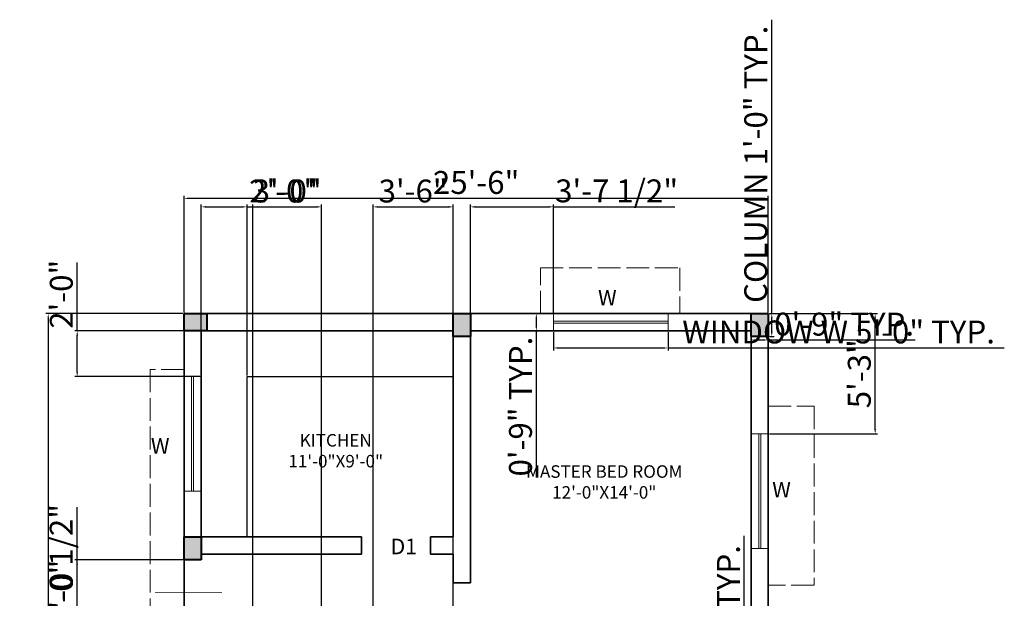
# Model space of a CAD drawing. Units: inches. Extents: x 27449 to 27965, y 46348 to 47103.
# Tile 2 of 2: x 27449 to 27965, y 46800 to 47103. Entities that reach past the tile are written whole.
import ezdxf

# ---------------------------------------------------------------- set-up
doc = ezdxf.new("R2010")
doc.units = ezdxf.units.IN
doc.linetypes.add('ACAD_ISO02W100', pattern=[15, 12, -3])
for name, color, linetype, lineweight in [('A-ANNO-DIMS', 2, 'Continuous', 18), ('A-ANNO-SYMB', 7, 'Continuous', 18), ('A-ANNO-TEXT', 7, 'Continuous', 18), ('A-AREA-IDEN', 7, 'Continuous', 20), ('A-COLS', 7, 'Continuous', 40), ('A-FLOR-FIXT', 9, 'Continuous', 25), ('A-GLAZ', 4, 'Continuous', 20), ('A-GLAZ-OVHD', 8, 'ACAD_ISO02W100', 13), ('A-WALL', 7, 'Continuous', 35)]:
    doc.layers.add(name, color=color, linetype=linetype, lineweight=lineweight)
doc.styles.get("Standard").update_dxf_attribs({"font": 'arial.ttf'})
doc.dimstyles.new('ISO-25', dxfattribs={"dimtxt": 12, "dimasz": 2.5, "dimexe": 1.25, "dimexo": 0.625, "dimtad": 1, "dimlunit": 3, "dimtxsty": 'Standard', "dimcen": 2.5, "dimadec": 0, "dimazin": 0, "dimtfac": 1, "dimtmove": 0, "dimatfit": 3, "dimfxl": 1, "dimarcsym": 0})

# ---------------------------------------------------------------- blocks, each defined once
blk = doc.blocks.new('*D1')
at = {"layer": 'A-ANNO-DIMS', "color": 0, "lineweight": -2, "transparency": 16777216}
for p, q in [((27534.79, 46948.86), (27463.05, 46948.86)), ((27464.3, 46946.36), (27464.3, 46393.36)), ((27534.79, 46390.86), (27463.05, 46390.86))]:
    blk.add_line(p, q, dxfattribs=at)
at = {"layer": 'A-ANNO-DIMS', "color": 0, "transparency": 16777216}
for points in [[(27463.88, 46946.36), (27464.71, 46946.36), (27464.3, 46948.86)], [(27463.88, 46393.36), (27464.71, 46393.36), (27464.3, 46390.86)]]:
    blk.add_solid(points, dxfattribs=at)
at = {"layer": 'Defpoints', "color": 0, "transparency": 16777216}
for p in [(27535.42, 46948.86), (27464.3, 46390.86), (27535.42, 46390.86)]:
    blk.add_point(p, dxfattribs=at)
at = {"layer": 'A-ANNO-DIMS', "color": 0, "transparency": 16777216, "insert": (27457.54, 46669.86), "char_height": 12, "attachment_point": 5, "rotation": 90}
blk.add_mtext('46\'-6"', dxfattribs=at)
blk = doc.blocks.new('*D2')
at = {"layer": 'A-ANNO-DIMS', "color": 0, "lineweight": -2, "transparency": 16777216}
for p, q in [((27535.42, 46949.49), (27535.42, 47010.55)), ((27841.42, 46949.49), (27841.42, 47010.55)), ((27537.92, 47009.3), (27838.92, 47009.3))]:
    blk.add_line(p, q, dxfattribs=at)
at = {"layer": 'A-ANNO-DIMS', "color": 0, "transparency": 16777216}
for points in [[(27537.92, 47009.72), (27537.92, 47008.88), (27535.42, 47009.3)], [(27838.92, 47009.72), (27838.92, 47008.88), (27841.42, 47009.3)]]:
    blk.add_solid(points, dxfattribs=at)
at = {"layer": 'Defpoints', "color": 0, "transparency": 16777216}
for p in [(27841.42, 47009.3), (27535.42, 46948.86), (27841.42, 46948.86)]:
    blk.add_point(p, dxfattribs=at)
at = {"layer": 'A-ANNO-DIMS', "color": 0, "transparency": 16777216, "insert": (27688.42, 47016.05), "char_height": 12, "attachment_point": 5}
blk.add_mtext('25\'-6"', dxfattribs=at)
blk = doc.blocks.new('WIN-W-60IN')
for p, q in [((0, 60), (9, 60)), ((0, 0), (0, 60)), ((4, 0), (4, 60)), ((5, 0), (5, 60)), ((9, 60), (9, 0)), ((9, 0), (0, 0))]:
    blk.add_line(p, q)
blk = doc.blocks.new('COL-9X12IN')
h = blk.add_hatch(color=256)
h.dxf.hatch_style = 1
h.paths.add_polyline_path([(9, 12), (0, 12), (0, 0), (9, 0)])
for p, q in [((0, 12), (9, 12)), ((0, 0), (0, 12)), ((9, 12), (9, 0)), ((9, 0), (0, 0))]:
    blk.add_line(p, q)
blk = doc.blocks.new('ENTRY-ARROW')
blk.add_lwpolyline([(0, 0, 0.5, 0.5, 0), (0, 22.23, 5, 0, 0), (0, 35.55, 0, 0, 0)], format="xyseb")
blk = doc.blocks.new('*D7')
at = {"layer": 'A-ANNO-DIMS', "color": 0, "lineweight": -2, "transparency": 16777216}
for p, q in [((27843.22, 46948.86), (27843.22, 47102.92)), ((27842.04, 46948.86), (27844.47, 46948.86)), ((27843.22, 46939.36), (27843.22, 46946.36)), ((27842.04, 46936.86), (27844.47, 46936.86))]:
    blk.add_line(p, q, dxfattribs=at)
at = {"layer": 'A-ANNO-DIMS', "color": 0, "transparency": 16777216}
for points in [[(27842.8, 46946.36), (27843.64, 46946.36), (27843.22, 46948.86)], [(27842.8, 46939.36), (27843.64, 46939.36), (27843.22, 46936.86)]]:
    blk.add_solid(points, dxfattribs=at)
at = {"layer": 'Defpoints', "color": 0, "transparency": 16777216}
for p in [(27841.42, 46948.86), (27843.22, 46948.86), (27841.42, 46936.86)]:
    blk.add_point(p, dxfattribs=at)
at = {"layer": 'A-ANNO-DIMS', "color": 0, "transparency": 16777216, "insert": (27836.39, 47027.14), "char_height": 12, "attachment_point": 5, "rotation": 90}
blk.add_mtext('COLUMN 1\'-0" TYP.', dxfattribs=at)
blk = doc.blocks.new('*D8')
at = {"layer": 'A-ANNO-DIMS', "color": 0, "lineweight": -2, "transparency": 16777216}
for p, q in [((27832.42, 46936.24), (27832.42, 46933.81)), ((27834.92, 46935.06), (27838.92, 46935.06)), ((27841.42, 46936.24), (27841.42, 46933.81)), ((27841.42, 46935.06), (27918.32, 46935.06))]:
    blk.add_line(p, q, dxfattribs=at)
at = {"layer": 'A-ANNO-DIMS', "color": 0, "transparency": 16777216}
for points in [[(27834.92, 46935.48), (27834.92, 46934.65), (27832.42, 46935.06)], [(27838.92, 46935.48), (27838.92, 46934.65), (27841.42, 46935.06)]]:
    blk.add_solid(points, dxfattribs=at)
at = {"layer": 'Defpoints', "color": 0, "transparency": 16777216}
for p in [(27832.42, 46936.86), (27841.42, 46936.86), (27841.42, 46935.06)]:
    blk.add_point(p, dxfattribs=at)
at = {"layer": 'A-ANNO-DIMS', "color": 0, "transparency": 16777216, "insert": (27881.12, 46941.81), "char_height": 12, "attachment_point": 5}
blk.add_mtext('0\'-9" TYP.', dxfattribs=at)
blk = doc.blocks.new('*D9')
at = {"layer": 'A-ANNO-DIMS', "color": 0, "lineweight": -2, "transparency": 16777216}
for p, q in [((27728.92, 46939.24), (27728.92, 46929.61)), ((27788.92, 46939.24), (27788.92, 46929.61)), ((27731.42, 46930.86), (27786.42, 46930.86)), ((27788.92, 46930.86), (27965, 46930.86))]:
    blk.add_line(p, q, dxfattribs=at)
at = {"layer": 'A-ANNO-DIMS', "color": 0, "transparency": 16777216}
for points in [[(27731.42, 46931.28), (27731.42, 46930.45), (27728.92, 46930.86)], [(27786.42, 46931.28), (27786.42, 46930.45), (27788.92, 46930.86)]]:
    blk.add_solid(points, dxfattribs=at)
at = {"layer": 'Defpoints', "color": 0, "transparency": 16777216}
for p in [(27728.92, 46939.86), (27788.92, 46939.86), (27788.92, 46930.86)]:
    blk.add_point(p, dxfattribs=at)
at = {"layer": 'A-ANNO-DIMS', "color": 0, "transparency": 16777216, "insert": (27878.21, 46937.7), "char_height": 12, "attachment_point": 5}
blk.add_mtext('WINDOW W 5\'-0" TYP.', dxfattribs=at)
blk = doc.blocks.new('*D10')
at = {"layer": 'A-ANNO-DIMS', "color": 0, "lineweight": -2, "transparency": 16777216}
for p, q in [((27728.29, 46948.86), (27718.67, 46948.86)), ((27719.92, 46946.36), (27719.92, 46942.36)), ((27728.29, 46939.86), (27718.67, 46939.86)), ((27719.92, 46939.86), (27719.92, 46862.97))]:
    blk.add_line(p, q, dxfattribs=at)
at = {"layer": 'A-ANNO-DIMS', "color": 0, "transparency": 16777216}
for points in [[(27719.5, 46946.36), (27720.34, 46946.36), (27719.92, 46948.86)], [(27719.5, 46942.36), (27720.34, 46942.36), (27719.92, 46939.86)]]:
    blk.add_solid(points, dxfattribs=at)
at = {"layer": 'Defpoints', "color": 0, "transparency": 16777216}
for p in [(27728.92, 46948.86), (27719.92, 46939.86), (27728.92, 46939.86)]:
    blk.add_point(p, dxfattribs=at)
at = {"layer": 'A-ANNO-DIMS', "color": 0, "transparency": 16777216, "insert": (27713.17, 46900.16), "char_height": 12, "attachment_point": 5, "rotation": 90}
blk.add_mtext('0\'-9" TYP.', dxfattribs=at)
blk = doc.blocks.new('*D11')
at = {"layer": 'A-ANNO-DIMS', "color": 0, "lineweight": -2, "transparency": 16777216}
for p, q in [((27828.82, 46689.61), (27828.82, 46832.34)), ((27831.79, 46689.61), (27827.57, 46689.61)), ((27828.82, 46668.11), (27828.82, 46687.11)), ((27831.79, 46665.61), (27827.57, 46665.61))]:
    blk.add_line(p, q, dxfattribs=at)
at = {"layer": 'A-ANNO-DIMS', "color": 0, "transparency": 16777216}
for points in [[(27828.4, 46687.11), (27829.24, 46687.11), (27828.82, 46689.61)], [(27828.4, 46668.11), (27829.24, 46668.11), (27828.82, 46665.61)]]:
    blk.add_solid(points, dxfattribs=at)
at = {"layer": 'Defpoints', "color": 0, "transparency": 16777216}
for p in [(27828.82, 46689.61), (27832.42, 46689.61), (27832.42, 46665.61)]:
    blk.add_point(p, dxfattribs=at)
at = {"layer": 'A-ANNO-DIMS', "color": 0, "transparency": 16777216, "insert": (27822.07, 46762.22), "char_height": 12, "attachment_point": 5, "rotation": 90}
blk.add_mtext('VENT V 2\'-0" TYP.', dxfattribs=at)
blk = doc.blocks.new('*D16')
at = {"layer": 'A-ANNO-DIMS', "color": 0, "lineweight": -2, "transparency": 16777216}
for p, q in [((27479.47, 46783.86), (27479.47, 46847.47)), ((27534.79, 46783.86), (27478.22, 46783.86)), ((27479.47, 46749.86), (27479.47, 46781.36)), ((27534.79, 46747.36), (27478.22, 46747.36))]:
    blk.add_line(p, q, dxfattribs=at)
at = {"layer": 'A-ANNO-DIMS', "color": 0, "transparency": 16777216}
for points in [[(27479.05, 46781.36), (27479.89, 46781.36), (27479.47, 46783.86)], [(27479.05, 46749.86), (27479.89, 46749.86), (27479.47, 46747.36)]]:
    blk.add_solid(points, dxfattribs=at)
at = {"layer": 'Defpoints', "color": 0, "transparency": 16777216}
for p in [(27479.47, 46783.86), (27535.42, 46783.86), (27535.42, 46747.36)]:
    blk.add_point(p, dxfattribs=at)
at = {"layer": 'A-ANNO-DIMS', "color": 0, "transparency": 16777216, "insert": (27472.64, 46816.91), "char_height": 12, "attachment_point": 5, "rotation": 90}
blk.add_mtext('3\'-0 1/2"', dxfattribs=at)
blk = doc.blocks.new('*D17')
at = {"layer": 'A-ANNO-DIMS', "color": 0, "lineweight": -2, "transparency": 16777216}
for p, q in [((27534.79, 46819.86), (27478.22, 46819.86)), ((27479.47, 46786.36), (27479.47, 46817.36)), ((27534.79, 46783.86), (27478.22, 46783.86))]:
    blk.add_line(p, q, dxfattribs=at)
at = {"layer": 'A-ANNO-DIMS', "color": 0, "transparency": 16777216}
for points in [[(27479.05, 46817.36), (27479.89, 46817.36), (27479.47, 46819.86)], [(27479.05, 46786.36), (27479.89, 46786.36), (27479.47, 46783.86)]]:
    blk.add_solid(points, dxfattribs=at)
at = {"layer": 'Defpoints', "color": 0, "transparency": 16777216}
for p in [(27479.47, 46819.86), (27535.42, 46819.86), (27535.42, 46783.86)]:
    blk.add_point(p, dxfattribs=at)
at = {"layer": 'A-ANNO-DIMS', "color": 0, "transparency": 16777216, "insert": (27472.71, 46801.86), "char_height": 12, "attachment_point": 5, "rotation": 90}
blk.add_mtext('3\'-0"', dxfattribs=at)
blk = doc.blocks.new('*D18')
at = {"layer": 'A-ANNO-DIMS', "color": 0, "lineweight": -2, "transparency": 16777216}
for p, q in [((27479.47, 46939.86), (27479.47, 46975.72)), ((27543.79, 46939.86), (27478.22, 46939.86)), ((27479.47, 46918.36), (27479.47, 46937.36)), ((27543.79, 46915.86), (27478.22, 46915.86))]:
    blk.add_line(p, q, dxfattribs=at)
at = {"layer": 'A-ANNO-DIMS', "color": 0, "transparency": 16777216}
for points in [[(27479.05, 46937.36), (27479.89, 46937.36), (27479.47, 46939.86)], [(27479.05, 46918.36), (27479.89, 46918.36), (27479.47, 46915.86)]]:
    blk.add_solid(points, dxfattribs=at)
at = {"layer": 'Defpoints', "color": 0, "transparency": 16777216}
for p in [(27479.47, 46939.86), (27544.42, 46939.86), (27544.42, 46915.86)]:
    blk.add_point(p, dxfattribs=at)
at = {"layer": 'A-ANNO-DIMS', "color": 0, "transparency": 16777216, "insert": (27472.72, 46959.04), "char_height": 12, "attachment_point": 5, "rotation": 90}
blk.add_mtext('2\'-0"', dxfattribs=at)
blk = doc.blocks.new('*D19')
at = {"layer": 'A-ANNO-DIMS', "color": 0, "lineweight": -2, "transparency": 16777216}
for p, q in [((27544.42, 46916.49), (27544.42, 47006.06)), ((27568.42, 46916.49), (27568.42, 47006.06)), ((27546.92, 47004.81), (27565.92, 47004.81)), ((27568.42, 47004.81), (27604.27, 47004.81))]:
    blk.add_line(p, q, dxfattribs=at)
at = {"layer": 'A-ANNO-DIMS', "color": 0, "transparency": 16777216}
for points in [[(27546.92, 47005.23), (27546.92, 47004.4), (27544.42, 47004.81)], [(27565.92, 47005.23), (27565.92, 47004.4), (27568.42, 47004.81)]]:
    blk.add_solid(points, dxfattribs=at)
at = {"layer": 'Defpoints', "color": 0, "transparency": 16777216}
for p in [(27568.42, 47004.81), (27544.42, 46915.86), (27568.42, 46915.86)]:
    blk.add_point(p, dxfattribs=at)
at = {"layer": 'A-ANNO-DIMS', "color": 0, "transparency": 16777216, "insert": (27587.6, 47011.56), "char_height": 12, "attachment_point": 5}
blk.add_mtext('2\'-0"', dxfattribs=at)
blk = doc.blocks.new('*D20')
at = {"layer": 'A-ANNO-DIMS', "color": 0, "lineweight": -2, "transparency": 16777216}
for p, q in [((27571.42, 46498.49), (27571.42, 47006.06)), ((27607.42, 46498.49), (27607.42, 47006.06)), ((27573.92, 47004.81), (27604.92, 47004.81))]:
    blk.add_line(p, q, dxfattribs=at)
at = {"layer": 'A-ANNO-DIMS', "color": 0, "transparency": 16777216}
for points in [[(27573.92, 47005.23), (27573.92, 47004.4), (27571.42, 47004.81)], [(27604.92, 47005.23), (27604.92, 47004.4), (27607.42, 47004.81)]]:
    blk.add_solid(points, dxfattribs=at)
at = {"layer": 'Defpoints', "color": 0, "transparency": 16777216}
for p in [(27607.42, 47004.81), (27571.42, 46497.86), (27607.42, 46497.86)]:
    blk.add_point(p, dxfattribs=at)
at = {"layer": 'A-ANNO-DIMS', "color": 0, "transparency": 16777216, "insert": (27589.42, 47011.57), "char_height": 12, "attachment_point": 5}
blk.add_mtext('3\'-0"', dxfattribs=at)
blk = doc.blocks.new('*D22')
at = {"layer": 'A-ANNO-DIMS', "color": 0, "lineweight": -2, "transparency": 16777216}
for p, q in [((27634.42, 46498.49), (27634.42, 47006.06)), ((27676.42, 46498.49), (27676.42, 47006.06)), ((27636.92, 47004.81), (27673.92, 47004.81))]:
    blk.add_line(p, q, dxfattribs=at)
at = {"layer": 'A-ANNO-DIMS', "color": 0, "transparency": 16777216}
for points in [[(27636.92, 47005.23), (27636.92, 47004.4), (27634.42, 47004.81)], [(27673.92, 47005.23), (27673.92, 47004.4), (27676.42, 47004.81)]]:
    blk.add_solid(points, dxfattribs=at)
at = {"layer": 'Defpoints', "color": 0, "transparency": 16777216}
for p in [(27676.42, 47004.81), (27634.42, 46497.86), (27676.42, 46497.86)]:
    blk.add_point(p, dxfattribs=at)
at = {"layer": 'A-ANNO-DIMS', "color": 0, "transparency": 16777216, "insert": (27655.42, 47011.57), "char_height": 12, "attachment_point": 5}
blk.add_mtext('3\'-6"', dxfattribs=at)
blk = doc.blocks.new('*D27')
at = {"layer": 'A-ANNO-DIMS', "color": 0, "lineweight": -2, "transparency": 16777216}
for p, q in [((27685.42, 46949.49), (27685.42, 47006.06)), ((27728.92, 46949.49), (27728.92, 47006.06)), ((27687.92, 47004.81), (27726.42, 47004.81)), ((27728.92, 47004.81), (27792.52, 47004.81))]:
    blk.add_line(p, q, dxfattribs=at)
at = {"layer": 'A-ANNO-DIMS', "color": 0, "transparency": 16777216}
for points in [[(27687.92, 47005.23), (27687.92, 47004.4), (27685.42, 47004.81)], [(27726.42, 47005.23), (27726.42, 47004.4), (27728.92, 47004.81)]]:
    blk.add_solid(points, dxfattribs=at)
at = {"layer": 'Defpoints', "color": 0, "transparency": 16777216}
for p in [(27728.92, 47004.81), (27685.42, 46948.86), (27728.92, 46948.86)]:
    blk.add_point(p, dxfattribs=at)
at = {"layer": 'A-ANNO-DIMS', "color": 0, "transparency": 16777216, "insert": (27761.97, 47011.65), "char_height": 12, "attachment_point": 5}
blk.add_mtext('3\'-7 1/2"', dxfattribs=at)
blk = doc.blocks.new('*D28')
at = {"layer": 'A-ANNO-DIMS', "color": 0, "lineweight": -2, "transparency": 16777216}
for p, q in [((27842.04, 46948.86), (27898.62, 46948.86)), ((27897.37, 46888.36), (27897.37, 46946.36)), ((27842.04, 46885.86), (27898.62, 46885.86))]:
    blk.add_line(p, q, dxfattribs=at)
at = {"layer": 'A-ANNO-DIMS', "color": 0, "transparency": 16777216}
for points in [[(27896.95, 46946.36), (27897.79, 46946.36), (27897.37, 46948.86)], [(27896.95, 46888.36), (27897.79, 46888.36), (27897.37, 46885.86)]]:
    blk.add_solid(points, dxfattribs=at)
at = {"layer": 'Defpoints', "color": 0, "transparency": 16777216}
for p in [(27841.42, 46948.86), (27897.37, 46948.86), (27841.42, 46885.86)]:
    blk.add_point(p, dxfattribs=at)
at = {"layer": 'A-ANNO-DIMS', "color": 0, "transparency": 16777216, "insert": (27890.61, 46917.36), "char_height": 12, "attachment_point": 5, "rotation": 90}
blk.add_mtext('5\'-3"', dxfattribs=at)

msp = doc.modelspace()

# ---------------------------------------------------------------- linework, layer by layer
at = {"layer": 'A-FLOR-FIXT'}
for p, q in [((27568.42, 46915.862), (27676.42, 46915.862)), ((27568.42, 46831.862), (27568.42, 46915.862))]:
    msp.add_line(p, q, dxfattribs=at)
at = {"layer": 'A-GLAZ-OVHD'}
for p, q in [((27722.063, 46948.862), (27722.063, 46972.862)), ((27722.063, 46972.862), (27795.101, 46972.862)), ((27795.101, 46972.862), (27795.101, 46948.862)), ((27535.42, 46919.634), (27517.698, 46919.634)), ((27517.698, 46919.634), (27517.698, 46673.583)), ((27841.42, 46900.323), (27865.42, 46900.323)), ((27865.42, 46900.323), (27865.42, 46806.516)), ((27865.42, 46806.516), (27841.42, 46806.516))]:
    msp.add_line(p, q, dxfattribs=at)
at = {"layer": 'A-WALL'}
for p, q in [((27535.42, 46948.862), (27841.42, 46948.862)), ((27535.42, 46819.862), (27535.42, 46948.862)), ((27685.42, 46807.862), (27685.42, 46948.862)), ((27841.42, 46948.862), (27841.42, 46390.862)), ((27544.42, 46939.862), (27676.42, 46939.862)), ((27544.42, 46831.862), (27544.42, 46939.862)), ((27676.42, 46831.862), (27676.42, 46939.862)), ((27685.42, 46939.862), (27832.42, 46939.862)), ((27832.42, 46939.862), (27832.42, 46771.862)), ((27544.42, 46831.862), (27628.42, 46831.862)), ((27628.42, 46831.862), (27628.42, 46822.862)), ((27664.42, 46831.862), (27664.42, 46822.862)), ((27664.42, 46831.862), (27676.42, 46831.862)), ((27535.42, 46390.862), (27535.42, 46819.862)), ((27544.42, 46822.862), (27628.42, 46822.862)), ((27544.42, 46819.862), (27544.42, 46822.862)), ((27664.42, 46822.862), (27676.42, 46822.862)), ((27676.42, 46807.862), (27676.42, 46822.862)), ((27685.42, 46807.862), (27676.42, 46807.862))]:
    msp.add_line(p, q, dxfattribs=at)

# ---------------------------------------------------------------- block references
at = {"layer": 'A-ANNO-SYMB', "rotation": 90}
msp.add_blockref('ENTRY-ARROW', (27555.331, 46802.797), dxfattribs=at)
at = {"layer": 'A-COLS', "rotation": 90.00000000005677}
msp.add_blockref('COL-9X12IN', (27547.42, 46939.862), dxfattribs=at)
at = {"layer": 'A-COLS'}
for p in [(27676.42, 46936.862), (27832.42, 46936.862), (27535.42, 46819.862)]:
    msp.add_blockref('COL-9X12IN', p, dxfattribs=at)
at = {"layer": 'A-GLAZ', "rotation": 270.0000000000313}
msp.add_blockref('WIN-W-60IN', (27728.92, 46948.862), dxfattribs=at)
at = {"layer": 'A-GLAZ'}
for p in [(27535.42, 46855.862), (27832.42, 46825.862)]:
    msp.add_blockref('WIN-W-60IN', p, dxfattribs=at)

# ---------------------------------------------------------------- texts
at = {"layer": 'A-ANNO-TEXT', "char_height": 8.14905, "attachment_point": 1}
for s, insert in [('{\\fTimes New Roman|b1|i0|c0|p18;W}', (27752.224, 46961.288)), ('{\\fTimes New Roman|b1|i0|c0|p18;W}', (27518.067, 46883.608)), ('{\\fTimes New Roman|b1|i0|c0|p18;W}', (27843.441, 46860.699)), ('{\\fTimes New Roman|b1|i0|c0|p18;D1}', (27643.607, 46830.914))]:
    msp.add_mtext_dynamic_manual_height_columns(s, width=8.14905, gutter_width=40.745, heights=[0], dxfattribs=dict(at, insert=insert))
at = {"layer": 'A-AREA-IDEN', "char_height": 6.55829, "attachment_point": 1}
for s, insert in [('\\pxqc;{\\fTimes New Roman|b1|i0|c0|p18;KITCHEN\\P11\'-0"X9\'-0"}', (27544.33, 46885.755)), ('\\pxqc;{\\fTimes New Roman|b1|i0|c0|p18;MASTER BED ROOM\\P12\'-0"X14\'-0"}', (27684.955, 46869.393))]:
    msp.add_mtext_dynamic_manual_height_columns(s, width=141.09002, gutter_width=32.791, heights=[0], dxfattribs=dict(at, insert=insert))

# ---------------------------------------------------------------- dimensions: what is measured, and where the dimension line sits
at = {"layer": 'A-ANNO-DIMS'}
for base, p1, p2, angle, text, picture, middle in [((27843.22, 46948.862), (27841.42, 46936.862), (27841.42, 46948.862), 90, 'COLUMN <> TYP.', '*D7', (27836.386, 47027.143)), ((27788.92, 46930.862), (27728.92, 46939.862), (27788.92, 46939.862), 0, 'WINDOW W <> TYP.', '*D9', (27878.21, 46937.696)), ((27719.92, 46939.862), (27728.92, 46948.862), (27728.92, 46939.862), 270, '<> TYP.', '*D10', (27713.168, 46900.164)), ((27828.82, 46689.612), (27832.42, 46665.612), (27832.42, 46689.612), 90, 'VENT V <> TYP.', '*D11', (27822.068, 46762.224))]:
    dim = msp.add_linear_dim(base=base, p1=p1, p2=p2, angle=angle, text=text, dimstyle='ISO-25', override={"dimdec": 1, "dimlfac": 1, "dimrnd": 0, "dimzin": 1, "dimdsep": 46, "dimlunit": 4, "dimfrac": 2}, dxfattribs=at)
    dim.commit()
    dim.dimension.update_dxf_attribs({"geometry": picture, "text_midpoint": middle})
for base, p1, p2, override, picture, middle in [((27728.92, 47004.812), (27685.42, 46948.862), (27728.92, 46948.862), {"dimdec": 1, "dimlfac": 1, "dimrnd": 0, "dimzin": 1, "dimdsep": 46, "dimlunit": 4, "dimfrac": 2}, '*D27', (27761.971, 47011.646)), ((27841.42, 47009.301), (27535.42, 46948.862), (27841.42, 46948.862), {"dimclrd": 0, "dimclre": 0, "dimclrt": 0}, '*D2', (27688.42, 47016.053)), ((27568.42, 47004.812), (27544.42, 46915.862), (27568.42, 46915.862), {"dimdec": 1, "dimlfac": 1, "dimrnd": 0, "dimzin": 1, "dimdsep": 46, "dimlunit": 4, "dimfrac": 2}, '*D19', (27587.597, 47011.564)), ((27607.42, 47004.812), (27571.42, 46497.862), (27607.42, 46497.862), {"dimdec": 1, "dimlfac": 1, "dimrnd": 0, "dimzin": 1, "dimdsep": 46, "dimlunit": 4, "dimfrac": 2}, '*D20', (27589.42, 47011.568)), ((27676.42, 47004.812), (27634.42, 46497.862), (27676.42, 46497.862), {"dimdec": 1, "dimlfac": 1, "dimrnd": 0, "dimzin": 1, "dimdsep": 46, "dimlunit": 4, "dimfrac": 2}, '*D22', (27655.42, 47011.568))]:
    dim = msp.add_linear_dim(base=base, p1=p1, p2=p2, dimstyle='ISO-25', override=override, dxfattribs=at)
    dim.commit()
    dim.dimension.update_dxf_attribs({"geometry": picture, "text_midpoint": middle})
for base, p1, p2, override, picture, middle in [((27479.47, 46939.862), (27544.42, 46915.862), (27544.42, 46939.862), {"dimdec": 1, "dimlfac": 1, "dimrnd": 0, "dimzin": 1, "dimdsep": 46, "dimlunit": 4, "dimfrac": 2}, '*D18', (27472.718, 46959.039)), ((27464.295, 46390.862), (27535.42, 46948.862), (27535.42, 46390.862), {"dimclrd": 0, "dimclre": 0, "dimclrt": 0}, '*D1', (27457.544, 46669.862)), ((27897.37, 46948.862), (27841.42, 46885.862), (27841.42, 46948.862), {"dimdec": 1, "dimlfac": 1, "dimrnd": 0, "dimzin": 1, "dimdsep": 46, "dimlunit": 4, "dimfrac": 2}, '*D28', (27890.614, 46917.362)), ((27479.47, 46783.862), (27535.42, 46747.362), (27535.42, 46783.862), {"dimdec": 1, "dimlfac": 1, "dimrnd": 0, "dimzin": 1, "dimdsep": 46, "dimlunit": 4, "dimfrac": 2}, '*D16', (27472.636, 46816.914)), ((27479.47, 46819.862), (27535.42, 46783.862), (27535.42, 46819.862), {"dimdec": 1, "dimlfac": 1, "dimrnd": 0, "dimzin": 1, "dimdsep": 46, "dimlunit": 4, "dimfrac": 2}, '*D17', (27472.714, 46801.862))]:
    dim = msp.add_linear_dim(base=base, p1=p1, p2=p2, angle=90, dimstyle='ISO-25', override=override, dxfattribs=at)
    dim.commit()
    dim.dimension.update_dxf_attribs({"geometry": picture, "text_midpoint": middle})
dim = msp.add_linear_dim(base=(27841.42, 46935.062), p1=(27832.42, 46936.862), p2=(27841.42, 46936.862), text='<> TYP.', dimstyle='ISO-25', override={"dimdec": 1, "dimlfac": 1, "dimrnd": 0, "dimzin": 1, "dimdsep": 46, "dimlunit": 4, "dimfrac": 2}, dxfattribs=at)
dim.commit()
dim.dimension.update_dxf_attribs({"geometry": '*D8', "text_midpoint": (27881.118, 46941.814)})

doc.saveas('drawing.dxf')
